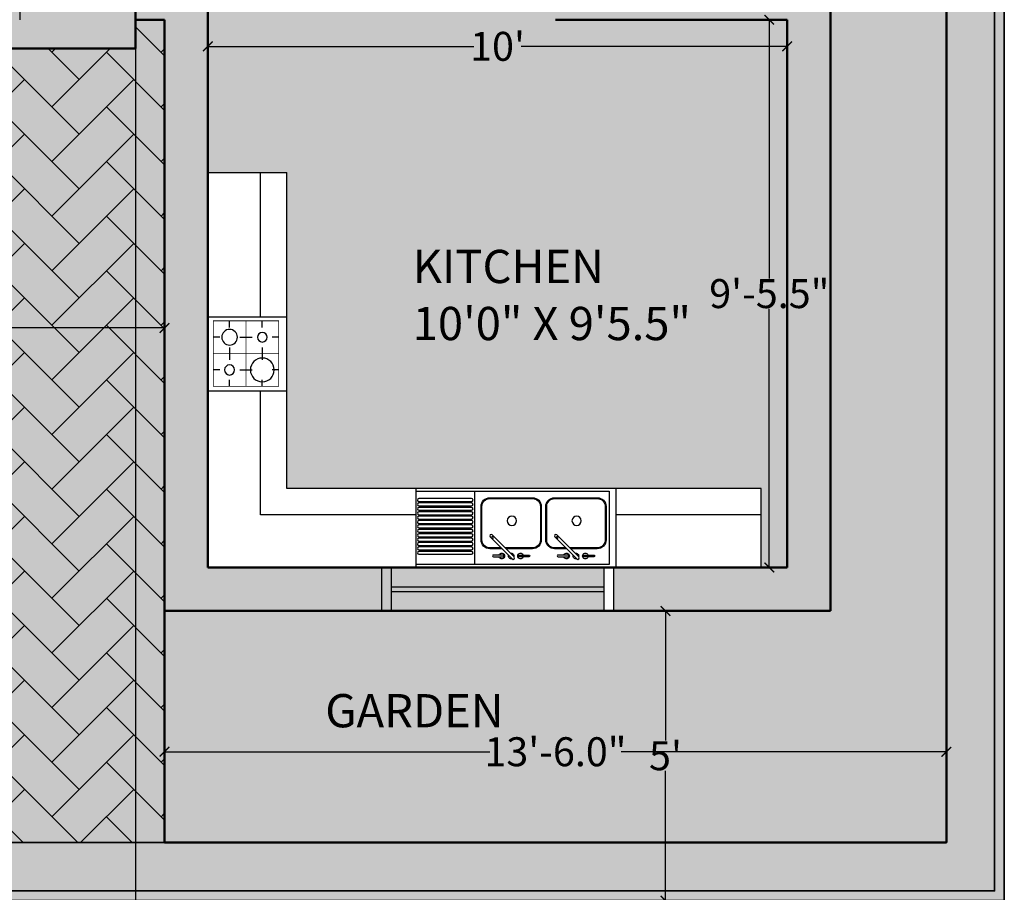
# Model space of a CAD drawing. Units: inches. Extents: x 528 to 2620, y -1066 to 798.
# Tile 3 of 41: x 740 to 944, y 211 to 391. Entities that reach past the tile are written whole.
import ezdxf

# ---------------------------------------------------------------- set-up
doc = ezdxf.new("R2010")
doc.units = ezdxf.units.IN
doc.header["$MEASUREMENT"] = 0
for name, color, linetype, lineweight in [('A-ANNO-DIMS', 2, 'Continuous', 18), ('A-AREA-IDEN', 7, 'Continuous', 18), ('A-Door', 2, 'Continuous', 25), ('A-FLOR-FIXT', 8, 'Continuous', 18), ('A-FLOR-PATT', 9, 'Continuous', 13), ('A-GLAZ', 3, 'Continuous', 25), ('A-WALL', 7, 'Continuous', 50), ('A-WALL-PATT', 8, 'Continuous', 13), ('C-PROP', 5, 'Continuous', 35)]:
    doc.layers.add(name, color=color, linetype=linetype, lineweight=lineweight)
doc.layers.add('TEFRIS', color=11, linetype='Continuous')
doc.styles.get("Standard").update_dxf_attribs({"font": 'arial.ttf'})
doc.dimstyles.get("Standard").update_dxf_attribs({"dimtxt": 6, "dimasz": 2, "dimexe": 0.18, "dimexo": 0.0625, "dimgap": 0.09, "dimtad": 0, "dimtih": 1, "dimtoh": 1, "dimdec": 1, "dimzin": 0, "dimdsep": 46, "dimlunit": 3, "dimtxsty": 'Standard', "dimblk": 'ARCHTICK', "dimcen": 0.09, "dimadec": 0, "dimazin": 0, "dimtfac": 1, "dimtdec": 1, "dimtofl": 0, "dimtmove": 0, "dimatfit": 3, "dimfxl": 1, "dimtolj": 1, "dimtzin": 0, "dimarcsym": 0})

# ---------------------------------------------------------------- blocks, each defined once
blk = doc.blocks.new('*U3')
for p, q in [((0, 0), (0, -6)), ((24, 0), (24, -6))]:
    blk.add_line(p, q)
blk.add_lwpolyline([(0, 0), (0, 24), (1.75, 24), (1.75, 0)], close=True)
blk.add_arc((0, 0), 24, 0, 90)
blk = doc.blocks.new('A$C2CE61BFE')
at = {"layer": 'TEFRIS'}
for p, q in [((12.72, 49.97), (12.72, 44.98)), ((37.56, 49.97), (37.56, 44.98)), ((5.3, 37.56), (0.31, 37.56)), ((20.47, 37.56), (29.81, 37.56)), ((49.97, 37.56), (44.98, 37.56)), ((12.72, 20.47), (12.72, 29.81)), ((37.56, 20.47), (37.56, 29.81)), ((5.3, 12.72), (0.31, 12.72)), ((20.47, 12.72), (29.81, 12.72)), ((49.97, 12.72), (44.98, 12.72)), ((12.72, 5.3), (12.72, 0.31)), ((37.56, 5.3), (37.56, 0.31))]:
    blk.add_line(p, q, dxfattribs=at)
at = {"layer": 'TEFRIS', "const_width": 0.617}
blk.add_lwpolyline([(49.97, 49.97), (0.31, 49.97), (0.31, 0.31), (49.97, 0.31)], close=True, dxfattribs=at)
at = {"layer": 'TEFRIS', "const_width": 0.514}
for points in [[(25.14, 49.97), (25.14, 0.31)], [(49.97, 25.14), (0.31, 25.14)]]:
    blk.add_lwpolyline(points, dxfattribs=at)
at = {"layer": 'TEFRIS'}
for centre, radius in [((37.56, 37.56), 9.04), ((12.72, 37.56), 3.83), ((12.72, 12.72), 5.97), ((37.56, 12.72), 3.62)]:
    blk.add_circle(centre, radius, dxfattribs=at)
blk = doc.blocks.new('A$C59F64124')
at = {"layer": 'TEFRIS'}
for p, q in [((0, 0), (0, 60)), ((146.83, 57.74), (0, 57.74)), ((44.54, 2.06), (44.54, 57.74)), ((146.83, 2.06), (146.83, 57.74)), ((0, 2.06), (146.83, 2.06))]:
    blk.add_line(p, q, dxfattribs=at)
for points in [[(56.35, 36.75), (73.1, 53.5, -1), (74.6, 52), (57.85, 35.25, -1)], [(105.52, 36.75), (122.27, 53.5, -1), (123.77, 52), (107.02, 35.25, -1)], [(58.87, 51.96), (66.5, 51.96, -0.563183), (66.5, 50.54), (58.87, 50.54, -1)], [(85.83, 51.96), (78.2, 51.96, 0.563183), (78.2, 50.54), (85.83, 50.54, 1)], [(108.04, 51.96), (115.67, 51.96, -0.563183), (115.67, 50.54), (108.04, 50.54, -1)], [(135, 51.96), (127.37, 51.96, 0.563183), (127.37, 50.54), (135, 50.54, 1)]]:
    blk.add_lwpolyline(points, format="xyb", close=True, dxfattribs=at)
for points in [[(2.23, 49.95), (42.31, 49.95, -1), (42.31, 47.72), (2.23, 47.72, -1), (2.23, 49.95)], [(2.23, 46.61), (42.31, 46.61, -1), (42.31, 44.38), (2.23, 44.38, -1), (2.23, 46.61)], [(65.32, 45.72), (56.17, 45.72, 0.414214), (49.49, 39.04)], [(49.49, 39.04), (49.49, 13.7, 0.414214), (56.17, 7.01), (88.58, 7.01, 0.414214), (95.26, 13.7), (95.26, 39.04, 0.414214), (88.58, 45.72), (68.32, 45.72, 0.414214)], [(64.66, 45.05), (56.17, 45.05, 0.414214), (50.15, 39.04)], [(50.15, 39.04), (50.15, 13.7, 0.414214), (56.17, 7.68), (88.58, 7.68, 0.414214), (94.6, 13.7), (94.6, 39.04, 0.414214), (88.58, 45.05), (67.66, 45.05, 0.414214)], [(114.49, 45.72), (105.34, 45.72, 0.414214), (98.65, 39.04)], [(98.65, 39.04), (98.65, 13.7, 0.414214), (105.34, 7.01), (137.75, 7.01, 0.414214), (144.43, 13.7), (144.43, 39.04, 0.414214), (137.75, 45.72), (117.49, 45.72, 0.330435)], [(113.83, 45.05), (105.34, 45.05, 0.414214), (99.32, 39.04)], [(99.32, 39.04), (99.32, 13.7, 0.414214), (105.34, 7.68), (137.75, 7.68, 0.414214), (143.77, 13.7), (143.77, 39.04, 0.414214), (137.75, 45.05), (116.83, 45.05, 0.333106)], [(2.23, 43.27), (42.31, 43.27, -1), (42.31, 41.04), (2.23, 41.04, -1), (2.23, 43.27)], [(2.23, 39.92), (42.31, 39.92, -1), (42.31, 37.7), (2.23, 37.7, -1), (2.23, 39.92)], [(2.23, 36.58), (42.31, 36.58, -1), (42.31, 34.36), (2.23, 34.36, -1), (2.23, 36.58)], [(2.23, 33.24), (42.31, 33.24, -1), (42.31, 31.02), (2.23, 31.02, -1), (2.23, 33.24)], [(2.23, 29.9), (42.31, 29.9, -1), (42.31, 27.68), (2.23, 27.68, -1), (2.23, 29.9)], [(2.23, 26.56), (42.31, 26.56, -1), (42.31, 24.34), (2.23, 24.34, -1), (2.23, 26.56)], [(2.23, 23.22), (42.31, 23.22, -1), (42.31, 20.99), (2.23, 20.99, -1), (2.23, 23.22)], [(2.23, 19.88), (42.31, 19.88, -1), (42.31, 17.65), (2.23, 17.65, -1), (2.23, 19.88)], [(2.23, 16.54), (42.31, 16.54, -1), (42.31, 14.31), (2.23, 14.31, -1), (2.23, 16.54)], [(2.23, 13.2), (42.31, 13.2, -1), (42.31, 10.97), (2.23, 10.97, -1), (2.23, 13.2)], [(2.23, 9.86), (42.31, 9.86, -1), (42.31, 7.63), (2.23, 7.63, -1), (2.23, 9.86)]]:
    blk.add_lwpolyline(points, format="xyb", dxfattribs=at)
for centre, radius in [((58.21, 37.11), 0.707), ((107.38, 37.11), 0.707), ((72.91, 24.51), 3.54), ((122.08, 24.51), 3.54)]:
    blk.add_circle(centre, radius, dxfattribs=at)
for centre, start, end in [((65.24, 51.25), 199.47122, 160.52878), ((72.35, 51.25), 75, 195), ((79.47, 51.25), 19.47122, 340.52878), ((114.41, 51.25), 199.47122, 160.52878), ((121.52, 51.25), 75, 195), ((128.64, 51.25), 19.47122, 340.52878), ((72.35, 51.25), 255, 15), ((121.52, 51.25), 255, 15)]:
    blk.add_arc(centre, 2.12, start, end, dxfattribs=at)
blk = doc.blocks.new('A$C344845E7')
at = {"layer": 'TEFRIS'}
for p, q in [((-0.6, 4.2), (-0.6, 0.6)), ((0, 4.2), (-0.6, 4.2)), ((-0.4, 4.2), (-0.4, 3.1)), ((0, 0), (0, 4.2)), ((0, 3.1), (-0.6, 3.1)), ((-0.4, 1.5788), (-0.4, 0.4)), ((-2.9993, 0), (-2.9993, 0.6)), ((-0.6, 0.6), (-2.9993, 0.6)), ((-1.9, 0.6), (-1.9, 0)), ((-1.3397, 0.6), (-1.3397, 0)), ((-1.9, 0.4), (-2.9993, 0.4)), ((-0.4, 0.4), (-1.3397, 0.4)), ((0, 0), (-2.9993, 0))]:
    blk.add_line(p, q, dxfattribs=at)
at = {"layer": 'TEFRIS', "xscale": -0.01, "yscale": 0.01, "zscale": 0.01, "rotation": 270}
for name, p in [('A$C59F64124', (-0.6, 1.5788)), ('A$C2CE61BFE', (-1.8756, 0.0373))]:
    blk.add_blockref(name, p, dxfattribs=at)
blk = doc.blocks.new('_ArchTick')
at = {"color": 0, "linetype": 'ByBlock', "const_width": 0.15}
blk.add_lwpolyline([(-0.5, -0.5), (0.5, 0.5)], dxfattribs=at)
blk = doc.blocks.new('*D15')
at = {"layer": 'A-ANNO-DIMS', "color": 0, "lineweight": -2, "transparency": 16777216}
for p, q in [((872.31, 268.92), (874.04, 268.92)), ((873.86, 268.92), (873.86, 242.06)), ((873.86, 208.92), (873.86, 235.78)), ((872.31, 208.92), (874.04, 208.92))]:
    blk.add_line(p, q, dxfattribs=at)
at = {"layer": 'Defpoints', "color": 0, "transparency": 16777216}
for p in [(872.24, 268.92), (872.24, 208.92), (873.86, 208.92)]:
    blk.add_point(p, dxfattribs=at)
at = {"layer": 'A-ANNO-DIMS', "color": 0, "lineweight": -2, "transparency": 16777216, "xscale": 2, "yscale": 2, "zscale": 2}
for p, rotation in [((873.86, 268.92), 90), ((873.86, 208.92), 270)]:
    blk.add_blockref('_ArchTick', p, dxfattribs=dict(at, rotation=rotation))
at = {"layer": 'A-ANNO-DIMS', "color": 0, "transparency": 16777216, "insert": (873.86, 238.92), "char_height": 6, "attachment_point": 5}
blk.add_mtext("\\A1;5'", dxfattribs=at)
blk = doc.blocks.new('*D16')
at = {"layer": 'A-ANNO-DIMS', "color": 0, "lineweight": -2, "transparency": 16777216}
for p, q in [((770.06, 239.57), (770.06, 239.93)), ((770.06, 239.75), (837.45, 239.75)), ((932.06, 239.75), (864.67, 239.75)), ((932.06, 239.57), (932.06, 239.93))]:
    blk.add_line(p, q, dxfattribs=at)
at = {"layer": 'Defpoints', "color": 0, "transparency": 16777216}
for p in [(770.06, 239.51), (932.06, 239.75), (932.06, 239.51)]:
    blk.add_point(p, dxfattribs=at)
at = {"layer": 'A-ANNO-DIMS', "color": 0, "lineweight": -2, "transparency": 16777216, "xscale": 2, "yscale": 2, "zscale": 2, "rotation": 180}
blk.add_blockref('_ArchTick', (770.06, 239.75), dxfattribs=at)
at = {"layer": 'A-ANNO-DIMS', "color": 0, "lineweight": -2, "transparency": 16777216, "xscale": 2, "yscale": 2, "zscale": 2}
blk.add_blockref('_ArchTick', (932.06, 239.75), dxfattribs=at)
at = {"layer": 'A-ANNO-DIMS', "color": 0, "transparency": 16777216, "insert": (851.06, 239.75), "char_height": 6, "attachment_point": 5}
blk.add_mtext('\\A1;13\'-6.0"', dxfattribs=at)
blk = doc.blocks.new('*D33')
at = {"layer": 'A-ANNO-DIMS', "color": 0, "lineweight": -2, "transparency": 16777216}
for p, q in [((896.35, 391.42), (895.19, 391.42)), ((895.37, 391.42), (895.37, 337.83)), ((895.37, 277.92), (895.37, 331.52)), ((896.35, 277.92), (895.19, 277.92))]:
    blk.add_line(p, q, dxfattribs=at)
at = {"layer": 'Defpoints', "color": 0, "transparency": 16777216}
for p in [(896.41, 391.42), (895.37, 277.92), (896.41, 277.92)]:
    blk.add_point(p, dxfattribs=at)
at = {"layer": 'A-ANNO-DIMS', "color": 0, "lineweight": -2, "transparency": 16777216, "xscale": 2, "yscale": 2, "zscale": 2}
for p, rotation in [((895.37, 391.42), 90), ((895.37, 277.92), 270)]:
    blk.add_blockref('_ArchTick', p, dxfattribs=dict(at, rotation=rotation))
at = {"layer": 'A-ANNO-DIMS', "color": 0, "transparency": 16777216, "insert": (895.37, 334.67), "char_height": 6, "attachment_point": 5}
blk.add_mtext('\\A1;9\'-5.5"', dxfattribs=at)
blk = doc.blocks.new('*D34')
at = {"layer": 'A-ANNO-DIMS', "color": 0, "lineweight": -2, "transparency": 16777216}
for p, q in [((779.06, 386.81), (779.06, 385.72)), ((779.06, 385.9), (834.16, 385.9)), ((899.06, 385.9), (843.96, 385.9)), ((899.06, 386.81), (899.06, 385.72))]:
    blk.add_line(p, q, dxfattribs=at)
at = {"layer": 'Defpoints', "color": 0, "transparency": 16777216}
for p in [(779.06, 386.87), (779.06, 385.9), (899.06, 386.87)]:
    blk.add_point(p, dxfattribs=at)
at = {"layer": 'A-ANNO-DIMS', "color": 0, "lineweight": -2, "transparency": 16777216, "xscale": 2, "yscale": 2, "zscale": 2, "rotation": 180}
blk.add_blockref('_ArchTick', (779.06, 385.9), dxfattribs=at)
at = {"layer": 'A-ANNO-DIMS', "color": 0, "lineweight": -2, "transparency": 16777216, "xscale": 2, "yscale": 2, "zscale": 2}
blk.add_blockref('_ArchTick', (899.06, 385.9), dxfattribs=at)
at = {"layer": 'A-ANNO-DIMS', "color": 0, "transparency": 16777216, "insert": (839.06, 385.9), "char_height": 6, "attachment_point": 5}
blk.add_mtext("\\A1;10'", dxfattribs=at)
blk = doc.blocks.new('*D37')
at = {"layer": 'A-ANNO-DIMS', "color": 0, "lineweight": -2, "transparency": 16777216}
for p, q in [((596.06, 330.11), (596.06, 327.39)), ((770.06, 330.11), (770.06, 327.39)), ((596.06, 327.57), (669.45, 327.57)), ((770.06, 327.57), (696.67, 327.57))]:
    blk.add_line(p, q, dxfattribs=at)
at = {"layer": 'Defpoints', "color": 0, "transparency": 16777216}
for p in [(596.06, 330.17), (770.06, 330.17), (596.06, 327.57)]:
    blk.add_point(p, dxfattribs=at)
at = {"layer": 'A-ANNO-DIMS', "color": 0, "lineweight": -2, "transparency": 16777216, "xscale": 2, "yscale": 2, "zscale": 2, "rotation": 180}
blk.add_blockref('_ArchTick', (596.06, 327.57), dxfattribs=at)
at = {"layer": 'A-ANNO-DIMS', "color": 0, "lineweight": -2, "transparency": 16777216, "xscale": 2, "yscale": 2, "zscale": 2}
blk.add_blockref('_ArchTick', (770.06, 327.57), dxfattribs=at)
at = {"layer": 'A-ANNO-DIMS', "color": 0, "transparency": 16777216, "insert": (683.06, 327.57), "char_height": 6, "attachment_point": 5}
blk.add_mtext('\\A1;14\'-6.0"', dxfattribs=at)
blk = doc.blocks.new('WIN-1200')
for p, q in [((677.56, 718.92), (725.56, 718.92)), ((677.56, 709.92), (677.56, 718.92)), ((679.56, 709.92), (679.56, 718.92)), ((723.56, 718.92), (723.56, 709.92)), ((725.56, 718.92), (725.56, 709.92)), ((679.56, 714.92), (723.56, 714.92)), ((679.56, 713.92), (723.56, 713.92)), ((725.56, 709.92), (677.56, 709.92))]:
    blk.add_line(p, q)
blk = doc.blocks.new('*D57')
at = {"layer": 'A-ANNO-DIMS', "color": 0, "lineweight": -2, "transparency": 16777216}
for p, q in [((716.06, 391.36), (716.06, 174.74)), ((764.06, 391.36), (764.06, 174.74)), ((716.06, 174.92), (731.87, 174.92)), ((764.06, 174.92), (748.24, 174.92))]:
    blk.add_line(p, q, dxfattribs=at)
at = {"layer": 'Defpoints', "color": 0, "transparency": 16777216}
for p in [(716.06, 391.42), (764.06, 391.42), (764.06, 174.92)]:
    blk.add_point(p, dxfattribs=at)
at = {"layer": 'A-ANNO-DIMS', "color": 0, "lineweight": -2, "transparency": 16777216, "xscale": 2, "yscale": 2, "zscale": 2, "rotation": 180}
blk.add_blockref('_ArchTick', (716.06, 174.92), dxfattribs=at)
at = {"layer": 'A-ANNO-DIMS', "color": 0, "lineweight": -2, "transparency": 16777216, "xscale": 2, "yscale": 2, "zscale": 2}
blk.add_blockref('_ArchTick', (764.06, 174.92), dxfattribs=at)
at = {"layer": 'A-ANNO-DIMS', "color": 0, "transparency": 16777216, "insert": (740.06, 174.92), "char_height": 6, "attachment_point": 5}
blk.add_mtext('\\A1;4\'-0"', dxfattribs=at)

msp = doc.modelspace()

# ---------------------------------------------------------------- hatches: boundary and pattern name
at = {"layer": 'A-FLOR-PATT', "transparency": 33554607}
h = msp.add_hatch(dxfattribs=at)
h.set_pattern_fill('AR-HBONE', color=256, scale=2)
h.paths.add_polyline_path([(770.06, 391.42), (764.06, 391.42), (764.06, 385.42), (716.06, 385.42), (716.06, 391.42), (620.06, 391.42), (596.06, 391.42), (596.06, 220.92), (770.06, 220.92), (770.06, 268.92)])
at = {"layer": 'A-WALL-PATT', "transparency": 33554687}
h = msp.add_hatch(color=256, dxfattribs=at)
h.dxf.hatch_style = 1
h.paths.add_polyline_path([(944.06, 753.92), (584.06, 753.92), (584.06, 208.92), (608.06, 208.92), (608.06, 210.92), (586.06, 210.92), (586.06, 751.92), (942.06, 751.92), (942.06, 210.92), (728.06, 210.92), (728.06, 208.92), (944.06, 208.92)])
h = msp.add_hatch(color=256, dxfattribs=at)
h.dxf.hatch_style = 1
h.paths.add_polyline_path([(942.06, 751.92), (586.06, 751.92), (586.06, 210.92), (608.06, 210.92), (608.06, 220.92), (596.06, 220.92), (596.06, 741.92), (932.06, 741.92), (932.06, 220.92), (770.06, 220.92), (728.06, 220.92), (728.06, 210.92), (942.06, 210.92)])
at = {"layer": 'A-WALL-PATT', "transparency": 33554475}
h = msp.add_hatch(color=256, dxfattribs=at)
h.dxf.hatch_style = 1
h.paths.add_polyline_path([(620.06, 718.92), (908.06, 718.92), (908.06, 268.92), (770.06, 268.92), (770.06, 220.92), (932.06, 220.92), (932.06, 741.92), (596.06, 741.92), (596.06, 391.42), (620.06, 391.42)])
at = {"layer": 'A-WALL-PATT', "transparency": 33554687}
h = msp.add_hatch(color=256, dxfattribs=at)
h.dxf.hatch_style = 1
h.paths.add_polyline_path([(861.06, 273.92), (817.06, 273.92), (817.06, 272.92), (861.06, 272.92)])
h.paths.add_polyline_path([(817.06, 277.92), (815.06, 277.92), (815.06, 268.92), (817.06, 268.92)])
h.paths.add_polyline_path([(908.06, 397.92), (899.06, 397.92), (899.06, 395.92), (908.06, 395.92)])
h.paths.add_polyline_path([(908.06, 443.92), (899.06, 443.92), (899.06, 441.92), (908.06, 441.92)])
h.paths.add_polyline_path([(904.06, 441.92), (903.06, 441.92), (903.06, 397.92), (904.06, 397.92)])
h.paths.add_polyline_path([(625.06, 561.42), (624.06, 561.42), (624.06, 537.42), (625.06, 537.42)])
h.paths.add_polyline_path([(648.75, 334.44), (720.04, 334.44), (720.04, 345), (648.75, 345)], flags=9)
h.paths.add_polyline_path([(819.73, 323.15), (880.33, 323.15), (880.33, 333.71), (819.73, 333.71)], flags=9)
h.paths.add_polyline_path([(779.9, 680.61), (821.76, 680.61), (821.76, 691.17), (779.9, 691.17)], flags=9)
h.paths.add_polyline_path([(779.88, 692.36), (817.14, 692.36), (817.14, 703.06), (779.88, 703.06)], flags=9)
h.paths.add_polyline_path([(799.99, 453.88), (860.59, 453.88), (860.59, 464.44), (799.99, 464.44)], flags=9)
h.paths.add_polyline_path([(650.87, 539.4), (708.78, 539.4), (708.78, 549.95), (650.87, 549.95)], flags=9)
h.paths.add_polyline_path([(788.5, 612.01), (849.1, 612.01), (849.1, 622.56), (788.5, 622.56)], flags=9)
h.paths.add_polyline_path([(639.54, 648.31), (700.13, 648.31), (700.13, 658.87), (639.54, 658.87)], flags=9)
h.paths.add_polyline_path([(648.91, 346.09), (747.71, 346.09), (747.71, 356.78), (648.91, 356.78)], flags=9)
h.paths.add_polyline_path([(676.86, 450.66), (746.74, 450.66), (746.74, 461.36), (676.86, 461.36)], flags=9)
h.paths.add_polyline_path([(819.71, 334.95), (865.53, 334.95), (865.53, 345.64), (819.71, 345.64)], flags=9)
h.paths.add_polyline_path([(806.3, 467.75), (874.05, 467.75), (874.05, 478.44), (806.3, 478.44)], flags=9)
h.paths.add_polyline_path([(653.23, 552.28), (690.5, 552.28), (690.5, 562.98), (653.23, 562.98)], flags=9)
h.paths.add_polyline_path([(789.9, 623.41), (843.21, 623.41), (843.21, 634.1), (789.9, 634.1)], flags=9)
h.paths.add_polyline_path([(639.77, 662.1), (693.08, 662.1), (693.08, 672.8), (639.77, 672.8)], flags=9)
h.paths.add_polyline_path([(801.59, 242.91), (846.33, 242.91), (846.33, 253.6), (801.59, 253.6)], flags=9)
h.paths.add_polyline_path([(925.36, 593.98), (925.36, 674.06), (914.67, 674.06), (914.67, 593.98)], flags=9)
h.paths.add_polyline_path([(612.56, 593.98), (612.56, 674.06), (601.87, 674.06), (601.87, 593.98)], flags=9)
h.paths.add_polyline_path([(723.31, 726.56), (803.39, 726.56), (803.39, 737.25), (723.31, 737.25)], flags=9)
at = {"layer": 'A-WALL-PATT', "transparency": 33554521}
h = msp.add_hatch(color=256, dxfattribs=at)
h.dxf.hatch_style = 1
h.paths.add_polyline_path([(629.06, 709.92), (677.56, 709.92), (677.56, 718.92), (620.06, 718.92), (620.06, 667.92), (629.06, 667.92)])
h.paths.add_polyline_path([(790.56, 718.92), (725.56, 718.92), (725.56, 709.92), (774.06, 709.92), (774.06, 577.92), (768.48, 577.92), (768.56, 573.42), (774.06, 573.42), (774.06, 567.42), (778.56, 567.42), (778.56, 669.42), (831.06, 669.42), (831.06, 675.92), (826.56, 675.92), (826.56, 673.92), (778.56, 673.92), (778.56, 709.92), (790.56, 709.92)])
h.paths.add_polyline_path([(908.06, 718.92), (879.06, 718.92), (879.06, 709.92), (899.06, 709.92), (899.06, 641.67), (908.06, 641.67)])
h.paths.add_polyline_path([(629.06, 619.92), (620.06, 619.92), (620.06, 561.42), (629.06, 561.42), (629.06, 573.42), (724.06, 573.42), (724.06, 569.42), (728.56, 569.42), (728.56, 577.92), (629.06, 577.92)])
h.paths.add_polyline_path([(779.06, 391.42), (779.06, 400.42), (770.06, 400.42), (764.06, 400.42), (764.06, 397.42), (764.06, 391.42), (770.06, 391.42), (770.06, 268.92), (815.06, 268.92), (815.06, 277.92), (779.06, 277.92), (779.06, 359.77)])
h.paths.add_polyline_path([(908.06, 395.92), (899.06, 395.92), (851.06, 395.92), (851.06, 391.42), (899.06, 391.42), (899.06, 277.92), (863.06, 277.92), (863.06, 268.92), (908.06, 268.92)])
h.paths.add_polyline_path([(908.06, 593.67), (899.06, 593.67), (899.06, 525.42), (778.56, 525.42), (778.56, 527.17), (774.06, 527.17), (774.06, 520.92), (899.06, 520.92), (899.06, 443.92), (908.06, 443.92)])
h.paths.add_polyline_path([(629.06, 520.92), (728.56, 520.92), (728.56, 545.42), (724.06, 545.42), (724.06, 525.42), (629.06, 525.42), (629.06, 537.42), (620.06, 537.42), (620.06, 484.67), (629.06, 484.67)])
h.paths.add_polyline_path([(629.06, 436.67), (620.06, 436.67), (620.06, 391.42), (648.56, 391.42), (648.56, 400.42), (629.06, 400.42)])
h.paths.add_polyline_path([(716.06, 397.42), (716.06, 400.42), (696.56, 400.42), (696.56, 391.42), (716.06, 391.42)])
at = {"layer": 'A-WALL-PATT', "transparency": 33554681}
h = msp.add_hatch(color=256, dxfattribs=at)
h.dxf.hatch_style = 1
h.paths.add_polyline_path([(629.06, 665.92), (625.06, 665.92), (625.06, 621.92), (629.06, 621.92)])
h.paths.add_polyline_path([(624.06, 665.92), (620.06, 665.92), (620.06, 621.92), (624.06, 621.92)])
h.paths.add_polyline_path([(723.56, 713.92), (679.56, 713.92), (679.56, 709.92), (723.56, 709.92)])
h.paths.add_polyline_path([(723.56, 718.92), (679.56, 718.92), (679.56, 714.92), (723.56, 714.92)])
h.paths.add_polyline_path([(814.56, 713.92), (790.56, 713.92), (790.56, 709.92), (814.56, 709.92)])
h.paths.add_polyline_path([(814.56, 718.92), (790.56, 718.92), (790.56, 714.92), (814.56, 714.92)])
h.paths.add_polyline_path([(877.06, 713.92), (833.06, 713.92), (833.06, 709.92), (877.06, 709.92)])
h.paths.add_polyline_path([(877.06, 718.92), (833.06, 718.92), (833.06, 714.92), (877.06, 714.92)])
h.paths.add_polyline_path([(908.06, 639.67), (904.06, 639.67), (904.06, 595.67), (908.06, 595.67)])
h.paths.add_polyline_path([(903.06, 639.67), (899.06, 639.67), (899.06, 595.67), (903.06, 595.67)])
h.paths.add_polyline_path([(908.06, 441.92), (904.06, 441.92), (904.06, 397.92), (908.06, 397.92)])
h.paths.add_polyline_path([(903.06, 441.92), (899.06, 441.92), (899.06, 397.92), (903.06, 397.92)])
h.paths.add_polyline_path([(861.06, 272.92), (817.06, 272.92), (817.06, 268.92), (861.06, 268.92)])
h.paths.add_polyline_path([(861.06, 277.92), (817.06, 277.92), (817.06, 273.92), (861.06, 273.92)])
h.paths.add_polyline_path([(694.56, 395.42), (650.56, 395.42), (650.56, 391.42), (694.56, 391.42)])
h.paths.add_polyline_path([(694.56, 400.42), (650.56, 400.42), (650.56, 396.42), (694.56, 396.42)])
h.paths.add_polyline_path([(629.06, 482.67), (625.06, 482.67), (625.06, 438.67), (629.06, 438.67)])
h.paths.add_polyline_path([(624.06, 482.67), (620.06, 482.67), (620.06, 438.67), (624.06, 438.67)])
h.paths.add_polyline_path([(629.06, 561.42), (625.06, 561.42), (625.06, 537.42), (629.06, 537.42)])
h.paths.add_polyline_path([(624.06, 561.42), (620.06, 561.42), (620.06, 537.42), (624.06, 537.42)])
at = {"layer": 'A-WALL-PATT', "transparency": 33554590}
h = msp.add_hatch(color=256, dxfattribs=at)
h.dxf.hatch_style = 1
h.paths.add_polyline_path([(774.06, 709.92), (629.06, 709.92), (629.06, 577.92), (728.56, 577.92), (728.56, 579.42), (728.56, 619.42), (730.31, 619.42), (730.31, 619.38, -0.401453), (768.56, 579.42), (768.56, 577.92), (774.06, 577.92)])
h.paths.add_polyline_path([(723.9, 686.06), (723.97, 686.06), (723.83, 686.13)], flags=0)
h.paths.add_polyline_path([(722.79, 642.7), (722.89, 642.76), (722.89, 684.99), (722.65, 685.24), (722.65, 685.82), (723.08, 686.26), (723.53, 686.26), (723.97, 686.06), (724.74, 686.13), (770.7, 686.13), (770.78, 686.14), (771.13, 686.27), (771.69, 686.09), (771.94, 685.48), (771.67, 684.9), (771.58, 684.87), (771.58, 642.78), (771.88, 642.51), (771.88, 641.92), (771.51, 641.46), (770.85, 641.46), (770.4, 641.83), (770.4, 641.55), (724.74, 641.55), (723.99, 641.7), (723.44, 641.41), (722.88, 641.59), (722.6, 642.14)], flags=16)
h.paths.add_polyline_path([(723.99, 641.7), (723.99, 641.71), (723.99, 641.7)], flags=0)
h.paths.add_polyline_path([(722.89, 642.73), (722.89, 684.99), (722.65, 685.24), (722.65, 685.82), (723.08, 686.26), (723.29, 686.26), (722.99, 686.17), (722.79, 685.97), (722.65, 685.68), (722.65, 685.43), (722.75, 685.14), (722.94, 684.94), (723.24, 684.81), (723.48, 684.81), (723.78, 684.9), (723.98, 685.1), (724.17, 685.49), (724.12, 685.64), (724.12, 685.25), (723.63, 684.75), (723.63, 642.96), (724.12, 642.51), (724.12, 641.89), (723.66, 641.46), (723.08, 641.46), (722.65, 641.9), (722.65, 642.48)], flags=0)
h.paths.add_polyline_path([(722.65, 642.29), (722.65, 642.04), (722.79, 641.75), (723.08, 641.46), (723.29, 641.46), (722.88, 641.59), (722.6, 642.14)], flags=0)
h.paths.add_polyline_path([(770.75, 686.13), (770.58, 686.13), (770.55, 686.06)], flags=0)
h.paths.add_polyline_path([(743.3, 645.29), (753.23, 659.4), (748.69, 663.75), (753.23, 668.54), (743.3, 682.46), (743.79, 682.59), (744.14, 682.68), (744.53, 682.93), (744.63, 683.08), (745.02, 683.33), (744.53, 684.07), (744.78, 684.16), (744.87, 684.31), (745.51, 684.4), (746.08, 684.65), (746.47, 684.65), (746.82, 684.81), (747.46, 685.03), (747.71, 685.14), (748.2, 685.28), (748.39, 685.52), (748.86, 685.52), (749.99, 686.13), (753.49, 676.03), (757.38, 680.15), (757.79, 679.76), (758.04, 680.65), (758.29, 681.23), (758.29, 682.05), (758.02, 682.59), (757.87, 683.17), (757.82, 683.78), (758.39, 684.07), (758.98, 684.2), (759.62, 684.16), (760.21, 683.96), (760.75, 683.67), (761.86, 683.67), (762.4, 683.96), (762.99, 684.11), (763.63, 684.11), (764.2, 683.96), (764.74, 683.67), (766.12, 683.67), (766.66, 683.96), (767.25, 684.16), (767.87, 684.2), (768.46, 684.07), (769.05, 683.78), (769, 683.17), (768.85, 682.59), (768.55, 682.05), (768.55, 681.23), (768.8, 680.65), (769.09, 679.75), (768.95, 678.83), (768.8, 678.23), (768.55, 677.65), (768.55, 676.82), (768.8, 676.24), (769.09, 675.34), (768.95, 674.42), (768.8, 673.82), (768.55, 673.28), (768.55, 672.41), (768.8, 671.87), (769, 671.29), (769.05, 670.64), (768.95, 670.02), (768.8, 669.41), (768.55, 668.87), (768.55, 668), (768.97, 667.24), (769.05, 666.28), (769.05, 665.56), (768.46, 665.32), (767.87, 665.16), (767.25, 665.16), (766.66, 665.36), (766.12, 665.7), (764.74, 665.7), (763.94, 665.2), (762.99, 665.2), (762.4, 665.36), (761.86, 665.7), (761, 665.7), (762.7, 664.09), (760.74, 662.03), (761.86, 662.03), (762.4, 662.32), (763.34, 662.55), (764.25, 662.32), (764.79, 662.03), (766.12, 662.03), (766.66, 662.32), (767.25, 662.52), (767.87, 662.56), (768.51, 662.43), (769.05, 662.12), (769.05, 661.4), (769.05, 660.8), (768.85, 660.21), (768.55, 659.68), (768.55, 658.85), (768.85, 658.27), (769, 657.66), (769.07, 656.75), (768.85, 655.85), (768.55, 655.27), (768.55, 654.44), (768.85, 653.86), (769.07, 652.96), (769, 652.05), (768.85, 651.44), (768.55, 650.91), (768.55, 650.03), (768.85, 649.5), (769, 648.91), (769.05, 648.26), (769, 647.64), (768.85, 647.03), (768.55, 646.5), (768.55, 645.62), (768.85, 645.09), (769.05, 644.55), (769.05, 643.9), (768.51, 643.65), (767.87, 643.52), (767.25, 643.52), (766.66, 643.72), (766.12, 644.06), (764.79, 644.06), (764.25, 643.72), (763.34, 643.49), (762.4, 643.72), (761.86, 644.06), (760.8, 644.06), (760.26, 643.72), (759.67, 643.52), (759.03, 643.52), (758.39, 643.65), (757.87, 643.9), (757.87, 644.55), (758.04, 645.09), (758.34, 645.62), (758.34, 646.5), (758.04, 647.03), (757.92, 647.64), (757.87, 648.06), (757.38, 647.59), (753.42, 651.77), (749.99, 641.62), (749.5, 641.71), (749.35, 641.95), (748.54, 642.45), (747.31, 642.94), (746.65, 642.94), (746.33, 643.18), (745.51, 643.57), (744.53, 643.65), (745.01, 644.4), (744.63, 644.64), (744.14, 644.89), (743.79, 645.13)], flags=0)
h.paths.add_polyline_path([(755.66, 654.93), (756.54, 654.69), (757.53, 654.33), (756.64, 654.58)], flags=0)
h.paths.add_polyline_path([(758.34, 649.2), (758.34, 648.71), (758.59, 644.3), (758.59, 648.8)], flags=0)
h.paths.add_polyline_path([(758.34, 649.29), (758.09, 649.7), (758.36, 649.17)], flags=0)
h.paths.add_polyline_path([(755.66, 672.79), (756.49, 673.04), (757.36, 673.35), (757.35, 673.36), (756.64, 673.15)], flags=0)
h.paths.add_polyline_path([(760.26, 639.64), (771.41, 639.64), (771.41, 624.04), (760.26, 624.04)], flags=16)
h.paths.add_polyline_path([(761.38, 638.53), (770.29, 638.53), (770.29, 625.15), (761.38, 625.15)], flags=0)
edge = h.paths.add_edge_path(flags=0)
edge.add_ellipse((765.84, 631.84), major_axis=(-2.24, 2.24), ratio=1, start_angle=-45, end_angle=45, ccw=False)
edge.add_ellipse((765.84, 631.84), major_axis=(-2.24, 2.24), ratio=1, start_angle=-135, end_angle=-45, ccw=False)
edge.add_ellipse((765.84, 631.84), major_axis=(-2.24, 2.24), ratio=1, start_angle=135, end_angle=-135, ccw=False)
edge.add_ellipse((765.84, 631.84), major_axis=(-2.24, 2.24), ratio=1, start_angle=45, end_angle=135, ccw=False)
h.paths.add_polyline_path([(758.59, 683.42), (758.59, 678.92), (758.37, 678.58), (758.34, 678.43), (758.09, 678.05), (758.34, 678.52), (758.34, 679.01)], flags=0)
h.paths.add_polyline_path([(760.26, 688.04), (760.26, 703.64), (771.41, 703.64), (771.41, 688.04)], flags=16)
h.paths.add_polyline_path([(770.4, 685.39), (770.4, 685.85), (770.85, 686.22), (771.51, 686.22), (771.88, 685.76), (771.88, 685.17), (771.58, 684.9), (771.58, 642.78), (771.88, 642.51), (771.88, 641.92), (771.51, 641.46), (770.85, 641.46), (770.4, 641.83), (770.4, 642.29)], flags=0)
h.paths.add_polyline_path([(770.53, 642.68), (771.05, 643.01), (771.67, 642.77), (771.94, 642.2), (771.69, 641.59), (771.13, 641.41), (770.55, 641.62), (770.35, 642.13)], flags=16)
h.paths.add_polyline_path([(761.38, 689.15), (761.38, 702.53), (770.29, 702.53), (770.29, 689.15)], flags=0)
edge = h.paths.add_edge_path(flags=0)
edge.add_ellipse((765.84, 695.84), major_axis=(2.24, 2.24), ratio=1, start_angle=405, end_angle=495, ccw=False)
edge.add_ellipse((765.84, 695.84), major_axis=(2.24, 2.24), ratio=1, start_angle=675, end_angle=765, ccw=False)
edge.add_ellipse((765.84, 695.84), major_axis=(2.24, 2.24), ratio=1, start_angle=585, end_angle=675, ccw=False)
edge.add_ellipse((765.84, 695.84), major_axis=(2.24, 2.24), ratio=1, start_angle=495, end_angle=585, ccw=False)
h.paths.add_polyline_path([(770.7, 684.9), (770.94, 684.74), (771.41, 684.74), (771.73, 685.03), (771.88, 685.34), (771.88, 685.64), (771.69, 686.09), (771.58, 686.13), (771.88, 685.76), (771.88, 685.17), (771.41, 684.74), (770.85, 684.74)], flags=0)
h.paths.add_polyline_path([(899.06, 709.92), (831.06, 709.92), (831.06, 699.92), (829.81, 699.92), (829.81, 675.92), (831.06, 675.92), (831.06, 669.42), (778.56, 669.42), (778.56, 567.17), (780.06, 567.17), (820.06, 567.17), (820.06, 565.42), (820.02, 565.42, -0.401453), (780.06, 527.17), (778.56, 527.17), (778.56, 525.42), (899.06, 525.42)])
h.paths.add_polyline_path([(849.2, 636.01), (849.27, 636.02), (849.13, 636.08)], flags=0)
h.paths.add_polyline_path([(848.19, 634.95), (847.95, 635.2), (847.95, 635.78), (848.38, 636.22), (848.83, 636.22), (849.27, 636.02), (850.04, 636.08), (896, 636.08), (896.08, 636.1), (896.43, 636.22), (896.99, 636.05), (897.24, 635.43), (896.97, 634.86), (896.88, 634.83), (896.88, 592.74), (897.18, 592.47), (897.18, 591.88), (896.81, 591.42), (896.15, 591.42), (895.7, 591.79), (895.7, 591.51), (850.04, 591.51), (849.29, 591.66), (848.74, 591.37), (848.18, 591.54), (847.9, 592.1), (848.09, 592.65), (848.19, 592.71)], flags=16)
h.paths.add_polyline_path([(849.29, 591.66), (849.29, 591.66), (849.29, 591.66)], flags=16)
h.paths.add_polyline_path([(848.19, 634.95), (847.95, 635.2), (847.95, 635.78), (848.38, 636.22), (848.59, 636.22), (848.29, 636.13), (848.09, 635.93), (847.95, 635.64), (847.95, 635.39), (848.05, 635.1), (848.24, 634.9), (848.54, 634.76), (848.78, 634.76), (849.08, 634.85), (849.28, 635.05), (849.47, 635.44), (849.42, 635.59), (849.42, 635.21), (848.93, 634.7), (848.93, 592.92), (849.42, 592.47), (849.42, 591.84), (848.96, 591.42), (848.38, 591.42), (847.95, 591.86), (847.95, 592.44), (848.19, 592.69)], flags=0)
h.paths.add_polyline_path([(847.95, 592.25), (847.95, 592), (848.09, 591.71), (848.38, 591.42), (848.59, 591.42), (848.18, 591.54), (847.9, 592.1)], flags=16)
h.paths.add_polyline_path([(896.05, 636.08), (895.88, 636.08), (895.85, 636.01)], flags=0)
h.paths.add_polyline_path([(868.6, 632.41), (869.09, 632.55), (869.44, 632.64), (869.83, 632.88), (869.93, 633.04), (870.32, 633.28), (869.83, 634.02), (870.08, 634.11), (870.17, 634.27), (870.81, 634.36), (871.38, 634.61), (871.77, 634.61), (872.12, 634.76), (872.76, 634.99), (873.01, 635.1), (873.5, 635.23), (873.69, 635.48), (874.16, 635.48), (875.29, 636.08), (878.79, 625.99), (882.68, 630.11), (883.09, 629.71), (883.34, 630.6), (883.59, 631.18), (883.59, 632.01), (883.32, 632.55), (883.17, 633.13), (883.12, 633.73), (883.69, 634.02), (884.28, 634.16), (884.92, 634.11), (885.51, 633.91), (886.05, 633.62), (887.16, 633.62), (887.7, 633.91), (888.29, 634.07), (888.93, 634.07), (889.5, 633.91), (890.04, 633.62), (891.42, 633.62), (891.96, 633.91), (892.55, 634.11), (893.17, 634.16), (893.76, 634.02), (894.35, 633.73), (894.3, 633.13), (894.15, 632.55), (893.85, 632.01), (893.85, 631.18), (894.1, 630.6), (894.39, 629.71), (894.25, 628.79), (894.1, 628.18), (893.85, 627.6), (893.85, 626.77), (894.1, 626.19), (894.39, 625.3), (894.25, 624.38), (894.1, 623.78), (893.85, 623.24), (893.85, 622.37), (894.1, 621.83), (894.3, 621.25), (894.35, 620.6), (894.25, 619.97), (894.1, 619.37), (893.85, 618.83), (893.85, 617.96), (894.27, 617.2), (894.35, 616.23), (894.35, 615.52), (893.76, 615.27), (893.17, 615.12), (892.55, 615.12), (891.96, 615.32), (891.42, 615.65), (890.04, 615.65), (889.25, 615.16), (888.29, 615.16), (887.7, 615.32), (887.16, 615.65), (886.31, 615.65), (888, 614.04), (886.04, 611.98), (887.16, 611.98), (887.7, 612.27), (888.64, 612.5), (889.55, 612.27), (890.09, 611.98), (891.42, 611.98), (891.96, 612.27), (892.55, 612.48), (893.17, 612.52), (893.81, 612.39), (894.35, 612.07), (894.35, 611.36), (894.35, 610.75), (894.15, 610.17), (893.85, 609.63), (893.85, 608.81), (894.15, 608.22), (894.3, 607.62), (894.37, 606.7), (894.15, 605.81), (893.85, 605.22), (893.85, 604.4), (894.15, 603.81), (894.37, 602.92), (894.3, 602), (894.15, 601.4), (893.85, 600.86), (893.85, 599.99), (894.15, 599.45), (894.3, 598.87), (894.35, 598.22), (894.3, 597.59), (894.15, 596.99), (893.85, 596.45), (893.85, 595.58), (894.15, 595.04), (894.35, 594.51), (894.35, 593.86), (893.81, 593.61), (893.17, 593.48), (892.55, 593.48), (891.96, 593.68), (891.42, 594.01), (890.09, 594.01), (889.55, 593.68), (888.64, 593.45), (887.7, 593.68), (887.16, 594.01), (886.1, 594.01), (885.56, 593.68), (884.97, 593.48), (884.33, 593.48), (883.69, 593.61), (883.17, 593.86), (883.17, 594.51), (883.34, 595.04), (883.64, 595.58), (883.64, 596.45), (883.34, 596.99), (883.22, 597.59), (883.17, 598.01), (882.68, 597.55), (878.72, 601.73), (875.29, 591.57), (874.8, 591.66), (874.65, 591.91), (873.84, 592.4), (872.61, 592.89), (871.95, 592.89), (871.63, 593.14), (870.81, 593.52), (869.83, 593.61), (870.31, 594.36), (869.93, 594.6), (869.44, 594.84), (869.09, 595.09), (868.6, 595.24), (878.53, 609.35), (873.99, 613.71), (878.53, 618.49)], flags=0)
h.paths.add_polyline_path([(880.96, 622.75), (881.79, 622.99), (882.66, 623.31), (882.65, 623.31), (881.94, 623.1)], flags=0)
h.paths.add_polyline_path([(880.96, 604.89), (881.84, 604.64), (882.83, 604.28), (881.94, 604.53)], flags=16)
h.paths.add_polyline_path([(883.39, 628.01), (883.64, 628.48), (883.64, 628.97), (883.89, 633.38), (883.89, 628.88), (883.67, 628.53), (883.64, 628.39)], flags=0)
h.paths.add_polyline_path([(883.64, 599.16), (883.64, 598.67), (883.89, 594.26), (883.89, 598.76)], flags=16)
h.paths.add_polyline_path([(883.64, 599.25), (883.39, 599.65), (883.66, 599.12)], flags=16)
h.paths.add_polyline_path([(885.56, 637.99), (885.56, 653.6), (896.71, 653.6), (896.71, 637.99)], flags=16)
h.paths.add_polyline_path([(885.56, 589.6), (896.71, 589.6), (896.71, 573.99), (885.56, 573.99)], flags=16)
h.paths.add_polyline_path([(886.68, 639.11), (886.68, 652.48), (895.59, 652.48), (895.59, 639.11)], flags=0)
h.paths.add_polyline_path([(886.68, 588.48), (895.59, 588.48), (895.59, 575.11), (886.68, 575.11)], flags=0)
edge = h.paths.add_edge_path(flags=0)
edge.add_ellipse((891.14, 645.79), major_axis=(2.24, 2.24), ratio=1, start_angle=405, end_angle=495, ccw=False)
edge.add_ellipse((891.14, 645.79), major_axis=(2.24, 2.24), ratio=1, start_angle=675, end_angle=765, ccw=False)
edge.add_ellipse((891.14, 645.79), major_axis=(2.24, 2.24), ratio=1, start_angle=585, end_angle=675, ccw=False)
edge.add_ellipse((891.14, 645.79), major_axis=(2.24, 2.24), ratio=1, start_angle=495, end_angle=585, ccw=False)
edge = h.paths.add_edge_path(flags=0)
edge.add_ellipse((891.14, 581.8), major_axis=(-2.24, 2.24), ratio=1, start_angle=-45, end_angle=45, ccw=False)
edge.add_ellipse((891.14, 581.8), major_axis=(-2.24, 2.24), ratio=1, start_angle=-135, end_angle=-45, ccw=False)
edge.add_ellipse((891.14, 581.8), major_axis=(-2.24, 2.24), ratio=1, start_angle=135, end_angle=-135, ccw=False)
edge.add_ellipse((891.14, 581.8), major_axis=(-2.24, 2.24), ratio=1, start_angle=45, end_angle=135, ccw=False)
h.paths.add_polyline_path([(895.7, 635.35), (895.7, 635.8), (896.15, 636.17), (896.81, 636.17), (897.18, 635.71), (897.18, 635.12), (896.88, 634.85), (896.88, 592.74), (897.18, 592.47), (897.18, 591.88), (896.81, 591.42), (896.15, 591.42), (895.7, 591.79), (895.7, 592.25)], flags=0)
h.paths.add_polyline_path([(896, 634.85), (896.24, 634.7), (896.71, 634.7), (897.03, 634.99), (897.18, 635.3), (897.18, 635.59), (896.99, 636.05), (896.88, 636.08), (897.18, 635.71), (897.18, 635.12), (896.71, 634.7), (896.15, 634.7)], flags=0)
h.paths.add_polyline_path([(895.83, 592.63), (896.35, 592.96), (896.97, 592.73), (897.24, 592.16), (896.99, 591.54), (896.43, 591.37), (895.85, 591.58), (895.65, 592.09)], flags=16)
h.paths.add_polyline_path([(725.25, 569.42), (724.06, 569.42), (724.06, 573.42), (629.06, 573.42), (629.06, 525.42), (724.06, 525.42), (724.06, 545.42), (725.25, 545.42)])
h.paths.add_polyline_path([(820.02, 565.42), (780.06, 565.42), (780.06, 567.17), (774.06, 567.17), (774.06, 567.42), (774.06, 573.42), (768.56, 573.42), (768.48, 577.92), (768.56, 577.92), (768.56, 579.42, 0.401453), (730.31, 619.38), (730.31, 579.42), (728.56, 579.42), (728.56, 573.42), (728.56, 569.42), (727.25, 569.42), (727.25, 545.42), (728.56, 545.42), (728.56, 520.92), (665.06, 520.92), (665.06, 436.42), (716.06, 436.42), (716.06, 421.42), (717.81, 421.42), (717.81, 421.36, -0.392996), (740.06, 397.42, -0.392996), (762.31, 421.36), (762.31, 421.42), (764.06, 421.42), (764.06, 400.42), (770.06, 400.42), (779.06, 400.42), (779.06, 391.42), (779.06, 359.77), (795.43, 359.77), (795.43, 294.3), (893.67, 294.3), (893.67, 277.92), (899.06, 277.92), (899.06, 391.42), (851.06, 391.42), (851.06, 395.92), (899.06, 395.92), (899.06, 443.92), (899.06, 520.92), (774.06, 520.92), (774.06, 527.17), (778.56, 527.17), (780.06, 527.17, 0.401453)])
h.paths.add_polyline_path([(774.06, 519.66), (842.12, 519.66), (842.12, 505.07), (788.64, 505.07), (788.64, 474.08), (788.64, 470.43, -0.883215), (779.53, 456.66), (774.97, 456.66, -0.414214), (774.06, 457.57)], flags=16)
h.paths.add_polyline_path([(775.88, 517.83), (840.3, 517.83), (840.3, 514.19), (788.64, 514.19), (788.64, 484.41), (779.53, 484.41), (779.53, 474.08), (775.88, 474.08)], flags=0)
h.paths.add_polyline_path([(706.7, 501.56, -0.254069), (706.7, 493.02), (698.31, 492.55), (698.31, 502.03)], flags=16)
h.paths.add_polyline_path([(691.33, 515.69), (691.8, 507.3), (682.32, 507.3), (682.79, 515.69, -0.254069)], flags=16)
h.paths.add_polyline_path([(695.49, 504.68), (695.49, 479.42), (678.64, 479.42), (678.64, 504.68)], flags=16)
h.paths.add_polyline_path([(706.7, 489.6, -0.254069), (706.7, 481.06), (698.31, 480.59), (698.31, 490.07)], flags=16)
h.paths.add_polyline_path([(675.81, 502.03), (675.81, 492.55), (667.42, 493.02, -0.254069), (667.42, 501.56)], flags=16)
h.paths.add_polyline_path([(691.8, 476.8), (691.33, 468.41, -0.254069), (682.79, 468.41), (682.32, 476.8)], flags=16)
h.paths.add_polyline_path([(675.81, 490.07), (675.81, 480.59), (667.42, 481.06, -0.254069), (667.42, 489.6)], flags=16)
h.paths.add_polyline_path([(764.06, 397.42), (762.31, 397.42), (762.31, 421.36, 0.392996), (740.06, 397.42, 0.392996), (717.81, 421.36), (717.81, 397.42), (716.06, 397.42), (716.06, 391.42), (716.06, 385.42), (764.06, 385.42), (764.06, 391.42)], flags=17)
h.paths.add_polyline_path([(716.06, 436.42), (705.86, 436.42), (705.86, 418.42), (716.06, 418.42), (716.06, 421.42)], flags=17)
h.paths.add_polyline_path([(716.06, 418.42), (705.86, 418.42), (705.86, 400.42), (716.06, 400.42)], flags=17)
h.paths.add_polyline_path([(705.86, 418.42), (695.66, 418.42), (695.66, 400.42), (696.56, 400.42), (705.86, 400.42)], flags=17)
h.paths.add_polyline_path([(705.86, 436.42), (695.66, 436.42), (695.66, 418.42), (705.86, 418.42)], flags=17)
h.paths.add_polyline_path([(695.66, 418.42), (685.46, 418.42), (685.46, 400.42), (695.66, 400.42)], flags=17)
h.paths.add_polyline_path([(695.66, 436.42), (685.46, 436.42), (685.46, 418.42), (695.66, 418.42)], flags=17)
h.paths.add_polyline_path([(685.46, 418.42), (675.26, 418.42), (675.26, 400.42), (685.46, 400.42)], flags=17)
h.paths.add_polyline_path([(685.46, 436.42), (675.26, 436.42), (675.26, 418.42), (685.46, 418.42)], flags=17)
h.paths.add_polyline_path([(675.26, 436.42), (665.06, 436.42), (665.06, 418.42), (675.26, 418.42)])
h.paths.add_polyline_path([(675.26, 418.42), (665.06, 418.42), (665.06, 400.42), (675.26, 400.42)])
h.paths.add_polyline_path([(665.06, 418.42), (646.97, 418.42), (646.99, 436.42), (629.06, 436.42), (629.06, 400.42), (665.06, 400.42)])
h.paths.add_polyline_path([(665.06, 436.42), (646.99, 436.42), (646.97, 418.42), (665.06, 418.42)], flags=17)
h.paths.add_polyline_path([(647.01, 446.62), (629.06, 446.62), (629.06, 436.67), (629.06, 436.42), (646.99, 436.42)])
h.paths.add_polyline_path([(665.06, 446.62), (647.01, 446.62), (646.99, 436.42), (665.06, 436.42)])
h.paths.add_polyline_path([(647.02, 456.82), (629.06, 456.82), (629.06, 446.62), (647.01, 446.62)])
h.paths.add_polyline_path([(665.06, 456.82), (647.02, 456.82), (647.01, 446.62), (665.06, 446.62)])
h.paths.add_polyline_path([(647.03, 467.02), (629.06, 467.02), (629.06, 456.82), (647.02, 456.82)])
h.paths.add_polyline_path([(665.06, 467.02), (647.03, 467.02), (647.02, 456.82), (665.06, 456.82)])
h.paths.add_polyline_path([(665.06, 477.22), (647.05, 477.22), (647.03, 467.02), (665.06, 467.02)])
h.paths.add_polyline_path([(647.05, 477.22), (629.06, 477.22), (629.06, 467.02), (647.03, 467.02)])
h.paths.add_polyline_path([(647.06, 487.22), (629.06, 487.22), (629.06, 477.22), (647.05, 477.22), (647.05, 479.02), (645.53, 483.25), (640.88, 480.37)])
h.paths.add_polyline_path([(665.06, 520.92), (629.06, 520.92), (629.06, 487.22), (647.06, 487.22), (665.06, 487.22)])
h.paths.add_polyline_path([(665.06, 487.22), (647.06, 487.22), (653.22, 480.35), (648.58, 483.24), (647.05, 479.02), (647.05, 477.22), (665.06, 477.22)])
at = {"layer": 'A-WALL-PATT', "transparency": 33554457}
h = msp.add_hatch(color=256, dxfattribs=at)
h.dxf.hatch_style = 1
h.paths.add_polyline_path([(770.06, 391.42), (764.06, 391.42), (764.06, 385.42), (716.06, 385.42), (716.06, 391.42), (620.06, 391.42), (596.06, 391.42), (596.06, 220.92), (770.06, 220.92), (770.06, 268.92)])

# ---------------------------------------------------------------- linework, layer by layer
at = {"layer": 'A-WALL'}
for p, q in [((932.06, 220.92), (932.06, 741.92)), ((908.06, 268.92), (908.06, 718.92)), ((764.06, 391.42), (764.06, 400.42)), ((779.06, 391.42), (779.06, 400.42)), ((770.06, 391.42), (764.06, 391.42)), ((764.06, 385.42), (764.06, 391.42)), ((764.06, 391.42), (770.06, 391.42)), ((770.06, 268.92), (770.06, 391.42)), ((770.06, 391.42), (770.06, 268.92)), ((779.06, 277.92), (779.06, 391.42)), ((899.06, 391.42), (851.06, 391.42)), ((899.06, 277.92), (899.06, 391.42)), ((716.06, 385.42), (764.06, 385.42)), ((779.06, 277.92), (899.06, 277.92)), ((770.06, 268.92), (908.06, 268.92)), ((770.06, 268.92), (770.06, 220.92)), ((770.06, 220.92), (932.06, 220.92))]:
    msp.add_line(p, q, dxfattribs=at)
at = {"layer": 'C-PROP'}
for points in [[(728.06, 208.92), (944.06, 208.92), (944.06, 753.92), (584.06, 753.92), (584.06, 208.92), (608.06, 208.92)], [(728.06, 210.92), (942.06, 210.92), (942.06, 751.92), (586.06, 751.92), (586.06, 210.92), (608.06, 210.92)]]:
    msp.add_lwpolyline(points, dxfattribs=at)
msp.add_lwpolyline([(596.06, 741.92), (596.06, 220.92), (932.06, 220.92), (932.06, 741.92)], close=True, dxfattribs=at)

# ---------------------------------------------------------------- block references
at = {"layer": 'A-Door'}
msp.add_blockref('*U3', (716.06, 397.42), dxfattribs=at)
at = {"layer": 'A-Door', "xscale": -1}
msp.add_blockref('*U3', (764.06, 397.42), dxfattribs=at)
at = {"layer": 'A-FLOR-FIXT', "xscale": 27.28801273268209, "yscale": 27.28801273268209, "zscale": 27.28801273268209, "rotation": 270}
msp.add_blockref('A$C344845E7', (779.06, 277.92), dxfattribs=at)
at = {"layer": 'A-GLAZ'}
msp.add_blockref('WIN-1200', (137.5, -441), dxfattribs=at)

# ---------------------------------------------------------------- texts
at = {"layer": 'A-AREA-IDEN'}
for s, height, p in [('KITCHEN', 6.891, (821.49, 336.85)), ('10\'0" X 9\'5.5"', 6.8907, (821.49, 325.03)), ('GARDEN', 6.891, (803.37, 244.81))]:
    msp.add_text(s, height=height, dxfattribs=at).set_placement(p)

# ---------------------------------------------------------------- dimensions: what is measured, and where the dimension line sits
at = {"layer": 'A-ANNO-DIMS'}
for base, p1, p2, picture, middle in [((895.37, 277.92), (896.41, 391.42), (896.41, 277.92), '*D33', (895.37, 334.67)), ((873.86, 208.92), (872.24, 268.92), (872.24, 208.92), '*D15', (873.86, 238.92))]:
    dim = msp.add_linear_dim(base=base, p1=p1, p2=p2, angle=90, dimstyle='Standard', override={"dimclrd": 0, "dimclre": 0, "dimclrt": 0}, dxfattribs=at)
    dim.commit()
    dim.dimension.update_dxf_attribs({"geometry": picture, "text_midpoint": middle})
for base, p1, p2, override, picture, middle in [((764.06, 174.92), (716.06, 391.42), (764.06, 391.42), {"dimdec": 1, "dimlfac": 1, "dimrnd": 0, "dimzin": 1, "dimdsep": 46, "dimlunit": 4, "dimfrac": 2}, '*D57', (740.06, 174.92)), ((779.06, 385.9), (899.06, 386.87), (779.06, 386.87), {"dimclrd": 0, "dimclre": 0, "dimclrt": 0}, '*D34', (839.06, 385.9)), ((596.06, 327.57), (770.06, 330.17), (596.06, 330.17), {"dimclrd": 0, "dimclre": 0, "dimclrt": 0}, '*D37', (683.06, 327.57)), ((932.06, 239.75), (770.06, 239.51), (932.06, 239.51), {"dimclrd": 0, "dimclre": 0, "dimclrt": 0}, '*D16', (851.06, 239.75))]:
    dim = msp.add_linear_dim(base=base, p1=p1, p2=p2, dimstyle='Standard', override=override, dxfattribs=at)
    dim.commit()
    dim.dimension.update_dxf_attribs({"geometry": picture, "text_midpoint": middle})

doc.saveas('drawing.dxf')
